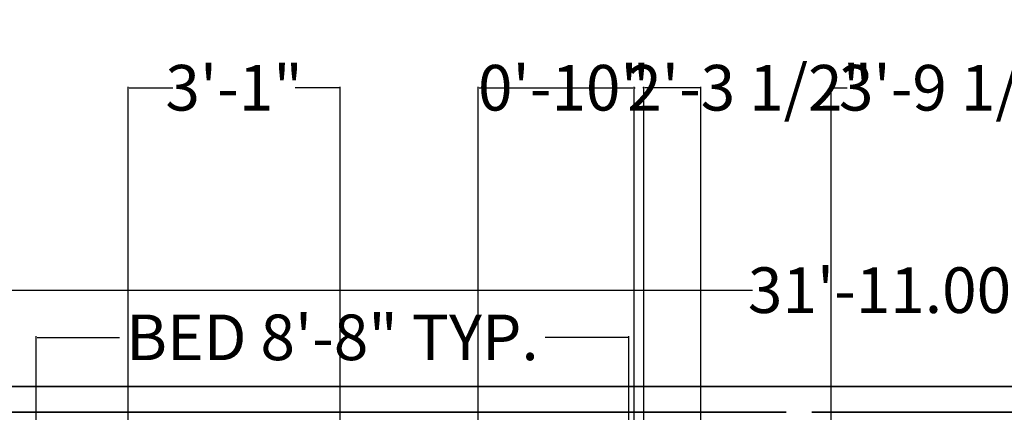
# Model space of a CAD drawing. Units: inches. Extents: x -438 to 102, y -60 to 1091.
# Tile 14 of 20: x -322 to -149, y 1022 to 1091. Entities that reach past the tile are written whole.
import ezdxf

# ---------------------------------------------------------------- set-up
doc = ezdxf.new("R2010")
doc.units = ezdxf.units.IN
doc.header["$MEASUREMENT"] = 0
for name, color, linetype, lineweight, true_color in [('A-ANNO-DIMS', 217, 'Continuous', 18, 0x93278f), ('A-WALL', 2, 'Continuous', 35, 0xf1eb1f), ('C-PROP', 2, 'Continuous', 35, 0xf1eb1f)]:
    doc.layers.add(name, color=color, linetype=linetype, lineweight=lineweight, true_color=true_color)
doc.styles.get("Standard").update_dxf_attribs({"font": 'arial.ttf'})
doc.dimstyles.get("Standard").update_dxf_attribs({"dimtxt": 8, "dimasz": 0.18, "dimexe": 0.18, "dimexo": 0.0625, "dimgap": 0.09, "dimtad": 0, "dimtih": 1, "dimtoh": 1, "dimdec": 4, "dimzin": 0, "dimdsep": 46, "dimlunit": 3, "dimtxsty": 'Standard', "dimcen": 0.09, "dimadec": 0, "dimazin": 0, "dimtfac": 1, "dimtdec": 4, "dimtofl": 0, "dimtmove": 0, "dimatfit": 3, "dimfxl": 1, "dimtolj": 1, "dimtzin": 0, "dimarcsym": 0})

# ---------------------------------------------------------------- blocks, each defined once
blk = doc.blocks.new('*D4')
at = {"layer": 'A-ANNO-DIMS', "color": 0, "lineweight": -2, "transparency": 16777216}
for p, q in [((-354.15, 1027.06), (-354.15, 1044.09)), ((-353.97, 1043.91), (-193.57, 1043.91)), ((28.67, 1043.91), (-131.73, 1043.91)), ((28.85, 1027.06), (28.85, 1044.09))]:
    blk.add_line(p, q, dxfattribs=at)
at = {"layer": 'A-ANNO-DIMS', "color": 0, "transparency": 16777216}
for points in [[(-353.97, 1043.94), (-353.97, 1043.88), (-354.15, 1043.91)], [(28.67, 1043.94), (28.67, 1043.88), (28.85, 1043.91)]]:
    blk.add_solid(points, dxfattribs=at)
at = {"layer": 'Defpoints', "color": 0, "transparency": 16777216}
for p in [(28.85, 1043.91), (-354.15, 1027), (28.85, 1027)]:
    blk.add_point(p, dxfattribs=at)
at = {"layer": 'A-ANNO-DIMS', "color": 0, "transparency": 16777216, "insert": (-162.65, 1043.91), "char_height": 8, "attachment_point": 5}
blk.add_mtext('\\A1;31\'-11.0000"', dxfattribs=at)
blk = doc.blocks.new('*D12')
at = {"layer": 'A-ANNO-DIMS', "color": 0, "lineweight": -2, "transparency": 16777216}
for p, q in [((-319.27, 1020.11), (-319.27, 1035.82)), ((-319.09, 1035.64), (-304.62, 1035.64)), ((-215.48, 1035.64), (-229.95, 1035.64)), ((-215.3, 1020.11), (-215.3, 1035.82))]:
    blk.add_line(p, q, dxfattribs=at)
at = {"layer": 'A-ANNO-DIMS', "color": 0, "transparency": 16777216}
for points in [[(-319.09, 1035.67), (-319.09, 1035.61), (-319.27, 1035.64)], [(-215.48, 1035.67), (-215.48, 1035.61), (-215.3, 1035.64)]]:
    blk.add_solid(points, dxfattribs=at)
at = {"layer": 'Defpoints', "color": 0, "transparency": 16777216}
for p in [(-215.3, 1035.64), (-319.27, 1020.04), (-215.3, 1020.04)]:
    blk.add_point(p, dxfattribs=at)
at = {"layer": 'A-ANNO-DIMS', "color": 0, "transparency": 16777216, "insert": (-267.28, 1035.64), "char_height": 8, "attachment_point": 5}
blk.add_mtext('\\A1;BED 8\'-8" TYP.', dxfattribs=at)
blk = doc.blocks.new('*D37')
at = {"layer": 'A-ANNO-DIMS', "color": 0, "lineweight": -2, "transparency": 16777216}
for p, q in [((-179.8, 234.94), (-179.8, 1079.58)), ((-179.62, 1079.4), (-176.98, 1079.4)), ((-134.26, 1079.4), (-136.9, 1079.4)), ((-134.08, 234.94), (-134.08, 1079.58))]:
    blk.add_line(p, q, dxfattribs=at)
at = {"layer": 'A-ANNO-DIMS', "color": 0, "transparency": 16777216}
for points in [[(-179.62, 1079.43), (-179.62, 1079.37), (-179.8, 1079.4)], [(-134.26, 1079.43), (-134.26, 1079.37), (-134.08, 1079.4)]]:
    blk.add_solid(points, dxfattribs=at)
at = {"layer": 'Defpoints', "color": 0, "transparency": 16777216}
for p in [(-134.08, 1079.4), (-179.8, 234.88), (-134.08, 234.88)]:
    blk.add_point(p, dxfattribs=at)
at = {"layer": 'A-ANNO-DIMS', "color": 0, "transparency": 16777216, "insert": (-156.94, 1079.4), "char_height": 8, "attachment_point": 5}
blk.add_mtext('\\A1;3\'-9 1/2"', dxfattribs=at)
blk = doc.blocks.new('*D41')
at = {"layer": 'A-ANNO-DIMS', "color": 0, "lineweight": -2, "transparency": 16777216}
for p, q in [((-303.15, 898.06), (-303.15, 1079.58)), ((-302.97, 1079.4), (-295.26, 1079.4)), ((-266.12, 1079.4), (-273.82, 1079.4)), ((-265.94, 898.06), (-265.94, 1079.58))]:
    blk.add_line(p, q, dxfattribs=at)
at = {"layer": 'A-ANNO-DIMS', "color": 0, "transparency": 16777216}
for points in [[(-302.97, 1079.43), (-302.97, 1079.37), (-303.15, 1079.4)], [(-266.12, 1079.43), (-266.12, 1079.37), (-265.94, 1079.4)]]:
    blk.add_solid(points, dxfattribs=at)
at = {"layer": 'Defpoints', "color": 0, "transparency": 16777216}
for p in [(-265.94, 1079.4), (-303.15, 898), (-265.94, 898)]:
    blk.add_point(p, dxfattribs=at)
at = {"layer": 'A-ANNO-DIMS', "color": 0, "transparency": 16777216, "insert": (-284.54, 1079.4), "char_height": 8, "attachment_point": 5}
blk.add_mtext('\\A1;3\'-1"', dxfattribs=at)
blk = doc.blocks.new('*D53')
at = {"layer": 'A-ANNO-DIMS', "color": 0, "lineweight": -2, "transparency": 16777216}
for p, q in [((-241.7, 824.44), (-241.7, 1079.58)), ((-241.52, 1079.4), (-214.55, 1079.4)), ((-214.37, 824.44), (-214.37, 1079.58)), ((-214.37, 1079.4), (-214.19, 1079.4))]:
    blk.add_line(p, q, dxfattribs=at)
at = {"layer": 'A-ANNO-DIMS', "color": 0, "transparency": 16777216}
for points in [[(-241.52, 1079.43), (-241.52, 1079.37), (-241.7, 1079.4)], [(-214.55, 1079.43), (-214.55, 1079.37), (-214.37, 1079.4)]]:
    blk.add_solid(points, dxfattribs=at)
at = {"layer": 'Defpoints', "color": 0, "transparency": 16777216}
for p in [(-214.37, 1079.4), (-241.7, 824.38), (-214.37, 824.38)]:
    blk.add_point(p, dxfattribs=at)
at = {"layer": 'A-ANNO-DIMS', "color": 0, "transparency": 16777216, "insert": (-194.08, 1079.4), "char_height": 8, "attachment_point": 5}
blk.add_mtext('\\A1;2\'-3 1/2"', dxfattribs=at)
blk = doc.blocks.new('*D61')
at = {"layer": 'A-ANNO-DIMS', "color": 0, "lineweight": -2, "transparency": 16777216}
for p, q in [((-212.65, 1079.4), (-212.83, 1079.4)), ((-212.65, 534.56), (-212.65, 1079.58)), ((-202.83, 1079.4), (-212.47, 1079.4)), ((-202.65, 534.56), (-202.65, 1079.58))]:
    blk.add_line(p, q, dxfattribs=at)
at = {"layer": 'A-ANNO-DIMS', "color": 0, "transparency": 16777216}
for points in [[(-212.47, 1079.43), (-212.47, 1079.37), (-212.65, 1079.4)], [(-202.83, 1079.43), (-202.83, 1079.37), (-202.65, 1079.4)]]:
    blk.add_solid(points, dxfattribs=at)
at = {"layer": 'Defpoints', "color": 0, "transparency": 16777216}
for p in [(-212.65, 1079.4), (-212.65, 534.5), (-202.65, 534.5)]:
    blk.add_point(p, dxfattribs=at)
at = {"layer": 'A-ANNO-DIMS', "color": 0, "transparency": 16777216, "insert": (-226.66, 1079.4), "char_height": 8, "attachment_point": 5}
blk.add_mtext('\\A1;0\'-10"', dxfattribs=at)

msp = doc.modelspace()

# ---------------------------------------------------------------- linework, layer by layer
at = {"layer": 'A-WALL'}
msp.add_line((-187.64649, 1022.49939), (-349.64649, 1022.49939), dxfattribs=at)
at = {"layer": 'C-PROP'}
for p, q in [((28.85351, 1026.99939), (-354.14649, 1026.99939)), ((-69.14649, 1022.49939), (-183.14649, 1022.49939))]:
    msp.add_line(p, q, dxfattribs=at)

# ---------------------------------------------------------------- dimensions: what is measured, and where the dimension line sits
at = {"layer": 'A-ANNO-DIMS'}
for base, p1, p2, override, picture, middle in [((-214.3672, 1079.39939), (-241.69558, 824.37939), (-214.3672, 824.37939), {"dimdec": 1, "dimlfac": 1, "dimrnd": 0, "dimzin": 1, "dimdsep": 46, "dimlunit": 4, "dimfrac": 2}, '*D53', (-194.07537, 1079.39939)), ((-134.07948, 1079.39939), (-179.79585, 234.87846), (-134.07948, 234.87846), {"dimdec": 1, "dimlfac": 1, "dimrnd": 0, "dimzin": 1, "dimdsep": 46, "dimlunit": 4, "dimfrac": 2}, '*D37', (-156.93767, 1079.39939)), ((-265.93641, 1079.39939), (-303.14649, 897.99939), (-265.93641, 897.99939), {"dimdec": 1, "dimlfac": 1, "dimrnd": 0, "dimzin": 1, "dimdsep": 46, "dimlunit": 4, "dimfrac": 2}, '*D41', (-284.54145, 1079.39939)), ((-212.64649, 1079.39939), (-202.64649, 534.49939), (-212.64649, 534.49939), {"dimdec": 1, "dimlfac": 1, "dimrnd": 0, "dimzin": 1, "dimdsep": 46, "dimlunit": 4, "dimfrac": 2}, '*D61', (-226.65728, 1079.39939)), ((28.85351, 1043.90502), (-354.14649, 1026.99939), (28.85351, 1026.99939), {"dimclrd": 0, "dimclre": 0, "dimclrt": 0}, '*D4', (-162.64649, 1043.90502))]:
    dim = msp.add_linear_dim(base=base, p1=p1, p2=p2, dimstyle='Standard', override=override, dxfattribs=at)
    dim.commit()
    dim.dimension.update_dxf_attribs({"geometry": picture, "text_midpoint": middle})
dim = msp.add_linear_dim(base=(-215.29994, 1035.63825), p1=(-319.26918, 1020.04286), p2=(-215.29994, 1020.04286), text='BED <> TYP.', dimstyle='Standard', override={"dimdec": 1, "dimlfac": 1, "dimrnd": 0, "dimzin": 1, "dimdsep": 46, "dimlunit": 4, "dimfrac": 2}, dxfattribs=at)
dim.commit()
dim.dimension.update_dxf_attribs({"geometry": '*D12', "text_midpoint": (-267.28456, 1035.63825)})

doc.saveas('drawing.dxf')
